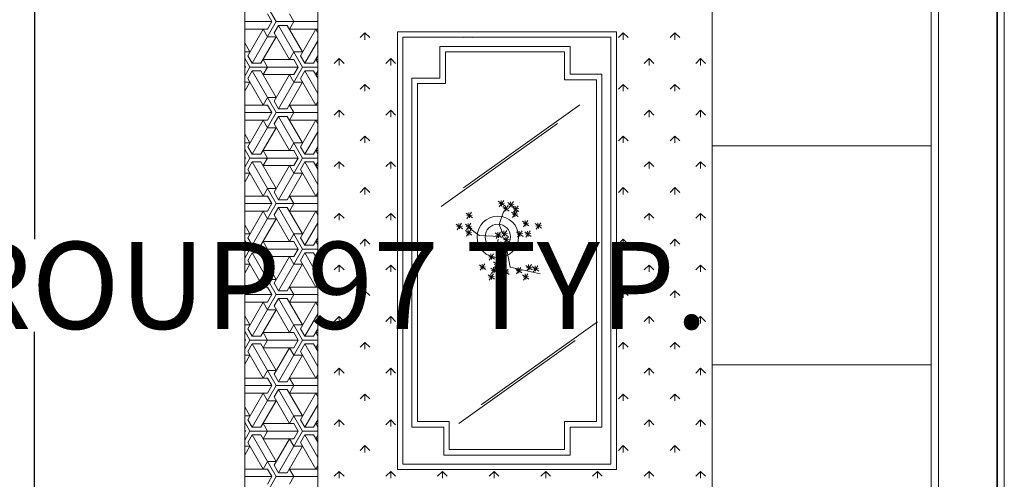
# Model space of a CAD drawing. Units: inches. Extents: x -1198 to -69, y -512 to 437.
# Tile 45 of 50: x -444 to -376, y 45 to 77. Entities that reach past the tile are written whole.
import ezdxf

# ---------------------------------------------------------------- set-up
doc = ezdxf.new("R2010")
doc.units = ezdxf.units.IN
doc.header["$MEASUREMENT"] = 0
for name, color, linetype, lineweight in [('A-ANNO-DIMS', 2, 'Continuous', 18), ('A-FURN', 60, 'Continuous', 18), ('A-WALL', 7, 'Continuous', 35)]:
    doc.layers.add(name, color=color, linetype=linetype, lineweight=lineweight)
doc.styles.get("Standard").update_dxf_attribs({"font": 'arial.ttf'})
doc.dimstyles.get("Standard").update_dxf_attribs({"dimtxt": 6, "dimasz": 6, "dimexe": 0.18, "dimexo": 0.0625, "dimgap": 0.09, "dimtad": 0, "dimtih": 1, "dimtoh": 1, "dimdec": 0, "dimzin": 0, "dimdsep": 46, "dimlunit": 4, "dimtxsty": 'Standard', "dimblk": 'OBLIQUE', "dimcen": 0.09, "dimadec": 0, "dimazin": 0, "dimtfac": 1, "dimtdec": 0, "dimtofl": 0, "dimtmove": 0, "dimatfit": 3, "dimfxl": 1, "dimtolj": 1, "dimtzin": 0, "dimarcsym": 0})

# ---------------------------------------------------------------- blocks, each defined once
blk = doc.blocks.new('A$C3B9F700E')
for p, q in [((736.9, 2080, -685.7), (2936.9, 2080, -685.7)), ((756.9, 2060, -685.7), (2916.9, 2060, -685.7)), ((2916.9, 1900, -685.7), (756.9, 1900, -685.7)), ((2936.9, 1880, -685.7), (736.9, 1880, -685.7)), ((2936.9, 1880, -685.7), (736.9, 1880, -685.7)), ((1536.9, 1880, -685.7), (1536.9, 1280, -685.7)), ((2136.9, 1880, -685.7), (2136.9, 1280, -685.7)), ((2736.9, 1280, -685.7), (936.9, 1280, -685.7)), ((1297.5, 1248.4, -685.7), (1310.8, 1261.7, -685.7)), ((1297.5, 1248.4, -685.7), (1310.8, 1235.2, -685.7)), ((1297.5, 1248.4, -685.7), (1316.3, 1248.4, -685.7)), ((1439, 1248.4, -685.7), (1452.2, 1261.7, -685.7)), ((1439, 1248.4, -685.7), (1452.2, 1235.2, -685.7)), ((1439, 1248.4, -685.7), (1457.7, 1248.4, -685.7)), ((1580.4, 1248.4, -685.7), (1593.6, 1261.7, -685.7)), ((1580.4, 1248.4, -685.7), (1593.6, 1235.2, -685.7)), ((1580.4, 1248.4, -685.7), (1599.1, 1248.4, -685.7)), ((1721.8, 1248.4, -685.7), (1735.1, 1261.7, -685.7)), ((1721.8, 1248.4, -685.7), (1735.1, 1235.2, -685.7)), ((1721.8, 1248.4, -685.7), (1740.6, 1248.4, -685.7)), ((1863.2, 1248.4, -685.7), (1876.5, 1261.7, -685.7)), ((1863.2, 1248.4, -685.7), (1876.5, 1235.2, -685.7)), ((1863.2, 1248.4, -685.7), (1882, 1248.4, -685.7)), ((2004.7, 1248.4, -685.7), (2017.9, 1261.7, -685.7)), ((2004.7, 1248.4, -685.7), (2017.9, 1235.2, -685.7)), ((2004.7, 1248.4, -685.7), (2023.4, 1248.4, -685.7)), ((2146.1, 1248.4, -685.7), (2159.3, 1261.7, -685.7)), ((2146.1, 1248.4, -685.7), (2159.3, 1235.2, -685.7)), ((2146.1, 1248.4, -685.7), (2164.8, 1248.4, -685.7)), ((2287.5, 1248.4, -685.7), (2300.8, 1261.7, -685.7)), ((2287.5, 1248.4, -685.7), (2300.8, 1235.2, -685.7)), ((2287.5, 1248.4, -685.7), (2306.2, 1248.4, -685.7)), ((2428.9, 1248.4, -685.7), (2442.2, 1261.7, -685.7)), ((2428.9, 1248.4, -685.7), (2442.2, 1235.2, -685.7)), ((2428.9, 1248.4, -685.7), (2447.7, 1248.4, -685.7)), ((1226.8, 1177.7, -685.7), (1240.1, 1191, -685.7)), ((1368.3, 1177.7, -685.7), (1381.5, 1191, -685.7)), ((1509.7, 1177.7, -685.7), (1522.9, 1191, -685.7)), ((1651.1, 1177.7, -685.7), (1664.4, 1191, -685.7)), ((1792.5, 1177.7, -685.7), (1805.8, 1191, -685.7)), ((1933.9, 1177.7, -685.7), (1947.2, 1191, -685.7)), ((2075.4, 1177.7, -685.7), (2088.6, 1191, -685.7)), ((2216.8, 1177.7, -685.7), (2230, 1191, -685.7)), ((2358.2, 1177.7, -685.7), (2371.5, 1191, -685.7)), ((1226.8, 1177.7, -685.7), (1240.1, 1164.5, -685.7)), ((1226.8, 1177.7, -685.7), (1245.6, 1177.7, -685.7)), ((1368.3, 1177.7, -685.7), (1381.5, 1164.5, -685.7)), ((1368.3, 1177.7, -685.7), (1387, 1177.7, -685.7)), ((1509.7, 1177.7, -685.7), (1522.9, 1164.5, -685.7)), ((1509.7, 1177.7, -685.7), (1528.4, 1177.7, -685.7)), ((1651.1, 1177.7, -685.7), (1664.4, 1164.5, -685.7)), ((1651.1, 1177.7, -685.7), (1669.9, 1177.7, -685.7)), ((1792.5, 1177.7, -685.7), (1805.8, 1164.5, -685.7)), ((1792.5, 1177.7, -685.7), (1811.3, 1177.7, -685.7)), ((1933.9, 1177.7, -685.7), (1947.2, 1164.5, -685.7)), ((1933.9, 1177.7, -685.7), (1952.7, 1177.7, -685.7)), ((2075.4, 1177.7, -685.7), (2088.6, 1164.5, -685.7)), ((2075.4, 1177.7, -685.7), (2094.1, 1177.7, -685.7)), ((2216.8, 1177.7, -685.7), (2230, 1164.5, -685.7)), ((2216.8, 1177.7, -685.7), (2235.5, 1177.7, -685.7)), ((2358.2, 1177.7, -685.7), (2371.5, 1164.5, -685.7)), ((2358.2, 1177.7, -685.7), (2377, 1177.7, -685.7)), ((1297.5, 1107, -685.7), (1310.8, 1120.3, -685.7)), ((1297.5, 1107, -685.7), (1310.8, 1093.8, -685.7)), ((1297.5, 1107, -685.7), (1316.3, 1107, -685.7)), ((1439, 1107, -685.7), (1452.2, 1120.3, -685.7)), ((1439, 1107, -685.7), (1452.2, 1093.8, -685.7)), ((1439, 1107, -685.7), (1457.7, 1107, -685.7)), ((1580.4, 1107, -685.7), (1593.6, 1120.3, -685.7)), ((1580.4, 1107, -685.7), (1593.6, 1093.8, -685.7)), ((1580.4, 1107, -685.7), (1599.1, 1107, -685.7)), ((1721.8, 1107, -685.7), (1735.1, 1120.3, -685.7)), ((1721.8, 1107, -685.7), (1735.1, 1093.8, -685.7)), ((1721.8, 1107, -685.7), (1740.6, 1107, -685.7)), ((1863.2, 1107, -685.7), (1876.5, 1120.3, -685.7)), ((1863.2, 1107, -685.7), (1876.5, 1093.8, -685.7)), ((1863.2, 1107, -685.7), (1882, 1107, -685.7)), ((2004.7, 1107, -685.7), (2017.9, 1120.3, -685.7)), ((2004.7, 1107, -685.7), (2017.9, 1093.8, -685.7)), ((2004.7, 1107, -685.7), (2023.4, 1107, -685.7)), ((2146.1, 1107, -685.7), (2159.3, 1120.3, -685.7)), ((2146.1, 1107, -685.7), (2159.3, 1093.8, -685.7)), ((2146.1, 1107, -685.7), (2164.8, 1107, -685.7)), ((2287.5, 1107, -685.7), (2300.8, 1120.3, -685.7)), ((2287.5, 1107, -685.7), (2300.8, 1093.8, -685.7)), ((2287.5, 1107, -685.7), (2306.2, 1107, -685.7)), ((2428.9, 1107, -685.7), (2442.2, 1120.3, -685.7)), ((2428.9, 1107, -685.7), (2442.2, 1093.8, -685.7)), ((2428.9, 1107, -685.7), (2447.7, 1107, -685.7)), ((1226.8, 1036.3, -685.7), (1240.1, 1049.6, -685.7)), ((1226.8, 1036.3, -685.7), (1240.1, 1023.1, -685.7)), ((1226.8, 1036.3, -685.7), (1245.6, 1036.3, -685.7)), ((1368.3, 1036.3, -685.7), (1381.5, 1049.6, -685.7)), ((1368.3, 1036.3, -685.7), (1381.5, 1023.1, -685.7)), ((1368.3, 1036.3, -685.7), (1387, 1036.3, -685.7)), ((1509.7, 1036.3, -685.7), (1522.9, 1049.6, -685.7)), ((1509.7, 1036.3, -685.7), (1522.9, 1023.1, -685.7)), ((1509.7, 1036.3, -685.7), (1528.4, 1036.3, -685.7)), ((1651.1, 1036.3, -685.7), (1664.4, 1049.6, -685.7)), ((1651.1, 1036.3, -685.7), (1664.4, 1023.1, -685.7)), ((1651.1, 1036.3, -685.7), (1669.9, 1036.3, -685.7)), ((1792.5, 1036.3, -685.7), (1805.8, 1049.6, -685.7)), ((1792.5, 1036.3, -685.7), (1805.8, 1023.1, -685.7)), ((1792.5, 1036.3, -685.7), (1811.3, 1036.3, -685.7)), ((1933.9, 1036.3, -685.7), (1947.2, 1049.6, -685.7)), ((1933.9, 1036.3, -685.7), (1947.2, 1023.1, -685.7)), ((1933.9, 1036.3, -685.7), (1952.7, 1036.3, -685.7)), ((2075.4, 1036.3, -685.7), (2088.6, 1049.6, -685.7)), ((2075.4, 1036.3, -685.7), (2088.6, 1023.1, -685.7)), ((2075.4, 1036.3, -685.7), (2094.1, 1036.3, -685.7)), ((2216.8, 1036.3, -685.7), (2230, 1049.6, -685.7)), ((2216.8, 1036.3, -685.7), (2230, 1023.1, -685.7)), ((2216.8, 1036.3, -685.7), (2235.5, 1036.3, -685.7)), ((2358.2, 1036.3, -685.7), (2371.5, 1049.6, -685.7)), ((2358.2, 1036.3, -685.7), (2371.5, 1023.1, -685.7)), ((2358.2, 1036.3, -685.7), (2377, 1036.3, -685.7)), ((1224, 417.9, -685.7), (1224, 1017.9, -685.7)), ((1224, 1017.9, -685.7), (2424, 1017.9, -685.7)), ((1239, 432.9, -685.7), (1239, 1002.9, -685.7)), ((1239, 1002.9, -685.7), (2409, 1002.9, -685.7)), ((2409, 1002.9, -685.7), (2409, 432.9, -685.7)), ((2424, 1017.9, -685.7), (2424, 417.9, -685.7)), ((1340.5, 977.9, -685.7), (2307.5, 977.9, -685.7)), ((1340.5, 890.9, -685.7), (1340.5, 977.9, -685.7)), ((2307.5, 977.9, -685.7), (2307.5, 890.9, -685.7)), ((2428.9, 965.6, -685.7), (2442.2, 978.9, -685.7)), ((1355.5, 962.9, -685.7), (2292.5, 962.9, -685.7)), ((1355.5, 875.9, -685.7), (1355.5, 962.9, -685.7)), ((2246, 647.2, -685.7), (2018.6, 965.9, -685.7)), ((2292.5, 962.9, -685.7), (2292.5, 875.9, -685.7)), ((2428.9, 965.6, -685.7), (2442.2, 952.3, -685.7)), ((2428.9, 965.6, -685.7), (2447.7, 965.6, -685.7)), ((1651.7, 598.7, -685.7), (1424.3, 917.3, -685.7)), ((1264, 534.4, -685.7), (1264, 890.9, -685.7)), ((1264, 890.9, -685.7), (1340.5, 890.9, -685.7)), ((2297.5, 586.5, -685.7), (2070.1, 905.2, -685.7)), ((2307.5, 890.9, -685.7), (2384, 890.9, -685.7)), ((2384, 890.9, -685.7), (2384, 544.9, -685.7)), ((1279, 549.4, -685.7), (1279, 875.9, -685.7)), ((1279, 875.9, -685.7), (1355.5, 875.9, -685.7)), ((2292.5, 875.9, -685.7), (2369, 875.9, -685.7)), ((2369, 875.9, -685.7), (2369, 559.9, -685.7)), ((1703.2, 538, -685.7), (1475.8, 856.6, -685.7)), ((2428.9, 824.2, -685.7), (2442.2, 837.4, -685.7)), ((1764.8, 797.9, -685.7), (1747.3, 810.4, -685.7)), ((1762.3, 812.9, -685.7), (1749.8, 795.4, -685.7)), ((1756.5, 797.3, -685.7), (1754.9, 812.4, -685.7)), ((1869.5, 726.5, -685.7), (1887, 808.9, -685.7)), ((2428.9, 824.2, -685.7), (2442.2, 810.9, -685.7)), ((2428.9, 824.2, -685.7), (2447.7, 824.2, -685.7)), ((1762.8, 804.4, -685.7), (1747.7, 802.8, -685.7)), ((1784.6, 784.3, -685.7), (1772.1, 766.8, -685.7)), ((1778.7, 768.6, -685.7), (1777.1, 783.7, -685.7)), ((1879.3, 772.4, -685.7), (1861.8, 784.9, -685.7)), ((1876.8, 787.4, -685.7), (1864.3, 769.9, -685.7)), ((1882.5, 790, -685.7), (1865, 802.5, -685.7)), ((1880.5, 796.5, -685.7), (1865.4, 794.9, -685.7)), ((1880, 805, -685.7), (1867.5, 787.5, -685.7)), ((1871, 771.8, -685.7), (1869.4, 786.9, -685.7)), ((1874.2, 789.3, -685.7), (1872.6, 804.4, -685.7)), ((1758.4, 762.9, -685.7), (1741, 775.4, -685.7)), ((1756.5, 769.4, -685.7), (1741.3, 767.8, -685.7)), ((1755.9, 777.9, -685.7), (1743.4, 760.4, -685.7)), ((1750.1, 762.2, -685.7), (1748.5, 777.4, -685.7)), ((1787.1, 769.3, -685.7), (1769.6, 781.8, -685.7)), ((1787.1, 747, -685.7), (1769.6, 759.5, -685.7)), ((1785.1, 775.8, -685.7), (1770, 774.2, -685.7)), ((1784.6, 762, -685.7), (1772.1, 744.5, -685.7)), ((1778.7, 746.3, -685.7), (1777.1, 761.4, -685.7)), ((1877.4, 779, -685.7), (1862.2, 777.4, -685.7)), ((1887.3, 743.8, -685.7), (1869.8, 756.3, -685.7)), ((1884.8, 758.8, -685.7), (1872.3, 741.3, -685.7)), ((1878.9, 743.1, -685.7), (1877.4, 758.3, -685.7)), ((1904.8, 762.9, -685.7), (1887.3, 775.4, -685.7)), ((1902.8, 769.4, -685.7), (1887.7, 767.8, -685.7)), ((1902.3, 777.9, -685.7), (1889.8, 760.4, -685.7)), ((1896.4, 762.2, -685.7), (1894.9, 777.4, -685.7)), ((1706.7, 723.1, -685.7), (1689.3, 735.6, -685.7)), ((1704.8, 729.6, -685.7), (1689.6, 728, -685.7)), ((1704.2, 738.1, -685.7), (1691.7, 720.6, -685.7)), ((1698.4, 722.4, -685.7), (1696.8, 737.6, -685.7)), ((1718.7, 735.8, -685.7), (1701.2, 748.3, -685.7)), ((1716.7, 742.3, -685.7), (1701.6, 740.7, -685.7)), ((1716.2, 750.8, -685.7), (1703.7, 733.3, -685.7)), ((1710.3, 735.2, -685.7), (1708.7, 750.3, -685.7)), ((1733, 733.4, -685.7), (1715.5, 745.9, -685.7)), ((1731, 740, -685.7), (1715.9, 738.4, -685.7)), ((1730.5, 748.4, -685.7), (1718, 730.9, -685.7)), ((1724.6, 732.8, -685.7), (1723.1, 747.9, -685.7)), ((1785.1, 753.5, -685.7), (1770, 751.9, -685.7)), ((1885.3, 750.3, -685.7), (1870.2, 748.7, -685.7)), ((1703.5, 696.8, -685.7), (1686.1, 709.3, -685.7)), ((1701.6, 703.3, -685.7), (1686.5, 701.7, -685.7)), ((1701, 711.8, -685.7), (1688.6, 694.3, -685.7)), ((1695.2, 696.2, -685.7), (1693.6, 711.3, -685.7)), ((1717.9, 708.8, -685.7), (1700.4, 721.3, -685.7)), ((1715.9, 715.3, -685.7), (1700.8, 713.7, -685.7)), ((1715.4, 723.8, -685.7), (1702.9, 706.3, -685.7)), ((1709.5, 708.1, -685.7), (1707.9, 723.2, -685.7)), ((1752.2, 696.5, -685.7), (1717.2, 709, -685.7)), ((1777.1, 706.5, -685.7), (1752.2, 696.5, -685.7)), ((1786.3, 704.8, -685.7), (1768.8, 717.3, -685.7)), ((1784.3, 711.3, -685.7), (1769.2, 709.7, -685.7)), ((1783.8, 719.8, -685.7), (1771.3, 702.3, -685.7)), ((1787.7, 703.1, -685.7), (1775.3, 685.6, -685.7)), ((1777.9, 704.1, -685.7), (1776.3, 719.3, -685.7)), ((1781.9, 687.4, -685.7), (1780.3, 702.5, -685.7)), ((1803, 709.6, -685.7), (1785.5, 722, -685.7)), ((1801, 716.1, -685.7), (1785.9, 714.5, -685.7)), ((1800.5, 724.5, -685.7), (1788, 707.1, -685.7)), ((1794.6, 708.9, -685.7), (1793, 724, -685.7)), ((1817.3, 689.7, -685.7), (1799.8, 702.1, -685.7)), ((1802.1, 714, -685.7), (1869.5, 726.5, -685.7)), ((1814.8, 704.6, -685.7), (1802.3, 687.2, -685.7)), ((1809, 689, -685.7), (1807.4, 704.1, -685.7)), ((1824.6, 689, -685.7), (1872, 714, -685.7)), ((1892, 708.8, -685.7), (1874.6, 721.3, -685.7)), ((1890.1, 715.3, -685.7), (1875, 713.7, -685.7)), ((1889.6, 723.8, -685.7), (1877.1, 706.3, -685.7)), ((1883.7, 708.1, -685.7), (1882.1, 723.2, -685.7)), ((1790.2, 688.1, -685.7), (1772.8, 700.6, -685.7)), ((1788.3, 694.6, -685.7), (1773.2, 693, -685.7)), ((1784.6, 699, -685.7), (1782.1, 641.6, -685.7)), ((1792.1, 694, -685.7), (1824.6, 689, -685.7)), ((1815.3, 696.2, -685.7), (1800.2, 694.6, -685.7)), ((1849.9, 669, -685.7), (1832.4, 681.5, -685.7)), ((1847.9, 675.5, -685.7), (1832.8, 673.9, -685.7)), ((1847.4, 683.9, -685.7), (1834.9, 666.5, -685.7)), ((1841.6, 668.3, -685.7), (1840, 683.4, -685.7)), ((1869.8, 684.1, -685.7), (1852.3, 696.6, -685.7)), ((1867.8, 690.6, -685.7), (1852.7, 689, -685.7)), ((1867.3, 699.1, -685.7), (1854.8, 681.6, -685.7)), ((1861.4, 683.4, -685.7), (1859.9, 698.6, -685.7)), ((1886.5, 676.1, -685.7), (1869, 688.6, -685.7)), ((1884.5, 682.6, -685.7), (1869.4, 681, -685.7)), ((1884, 691.1, -685.7), (1871.5, 673.6, -685.7)), ((1878.1, 675.5, -685.7), (1876.6, 690.6, -685.7)), ((1904.8, 669, -685.7), (1887.3, 681.5, -685.7)), ((1902.8, 675.5, -685.7), (1887.7, 673.9, -685.7)), ((1902.3, 683.9, -685.7), (1889.8, 666.5, -685.7)), ((1896.4, 668.3, -685.7), (1894.9, 683.4, -685.7)), ((2428.9, 682.8, -685.7), (2442.2, 696, -685.7)), ((2428.9, 682.8, -685.7), (2442.2, 669.5, -685.7)), ((2428.9, 682.8, -685.7), (2447.7, 682.8, -685.7)), ((1877.7, 645.1, -685.7), (1860.3, 657.6, -685.7)), ((1875.8, 651.6, -685.7), (1860.7, 650, -685.7)), ((1875.2, 660.1, -685.7), (1862.8, 642.6, -685.7)), ((1869.4, 644.4, -685.7), (1867.8, 659.5, -685.7)), ((1239, 624.2, -685.7), (1240.1, 625.3, -685.7)), ((1736.2, 608.5, -685.7), (1718.7, 621, -685.7)), ((1733.7, 623.4, -685.7), (1721.2, 606, -685.7)), ((1727.8, 607.8, -685.7), (1726.2, 622.9, -685.7)), ((1763.9, 621.9, -685.7), (1751.4, 604.4, -685.7)), ((1758, 606.2, -685.7), (1756.5, 621.3, -685.7)), ((1782.1, 641.6, -685.7), (1759.7, 611.6, -685.7)), ((1781.4, 621.9, -685.7), (1768.9, 604.4, -685.7)), ((1775.5, 606.2, -685.7), (1774, 621.3, -685.7)), ((1239, 599.9, -685.7), (1240.1, 598.8, -685.7)), ((1734.2, 615, -685.7), (1719.1, 613.4, -685.7)), ((1766.4, 606.9, -685.7), (1748.9, 619.4, -685.7)), ((1766.4, 581.4, -685.7), (1748.9, 593.9, -685.7)), ((1764.4, 613.4, -685.7), (1749.3, 611.8, -685.7)), ((1763.9, 596.4, -685.7), (1751.4, 578.9, -685.7)), ((1758, 580.7, -685.7), (1756.5, 595.9, -685.7)), ((1783.9, 606.9, -685.7), (1766.4, 619.4, -685.7)), ((1781.9, 613.4, -685.7), (1766.8, 611.8, -685.7)), ((1764.4, 587.9, -685.7), (1749.3, 586.3, -685.7)), ((1366, 549.4, -685.7), (1279, 549.4, -685.7)), ((1366, 472.9, -685.7), (1366, 549.4, -685.7)), ((2292.5, 559.9, -685.7), (2292.5, 472.9, -685.7)), ((2369, 559.9, -685.7), (2292.5, 559.9, -685.7)), ((2307.5, 544.9, -685.7), (2307.5, 457.9, -685.7)), ((2384, 544.9, -685.7), (2307.5, 544.9, -685.7)), ((2428.9, 541.3, -685.7), (2442.2, 554.6, -685.7)), ((2428.9, 541.3, -685.7), (2442.2, 528.1, -685.7)), ((2428.9, 541.3, -685.7), (2447.7, 541.3, -685.7)), ((1351, 534.4, -685.7), (1264, 534.4, -685.7)), ((1351, 457.9, -685.7), (1351, 534.4, -685.7)), ((2292.5, 472.9, -685.7), (1366, 472.9, -685.7)), ((2409, 432.9, -685.7), (1239, 432.9, -685.7)), ((2307.5, 457.9, -685.7), (1351, 457.9, -685.7)), ((2424, 417.9, -685.7), (1224, 417.9, -685.7)), ((1297.5, 399.9, -685.7), (1310.8, 413.2, -685.7)), ((1439, 399.9, -685.7), (1452.2, 413.2, -685.7)), ((1580.4, 399.9, -685.7), (1593.6, 413.2, -685.7)), ((1721.8, 399.9, -685.7), (1735.1, 413.2, -685.7)), ((1863.2, 399.9, -685.7), (1876.5, 413.2, -685.7)), ((2004.7, 399.9, -685.7), (2017.9, 413.2, -685.7)), ((2146.1, 399.9, -685.7), (2159.3, 413.2, -685.7)), ((2287.5, 399.9, -685.7), (2300.8, 413.2, -685.7)), ((2428.9, 399.9, -685.7), (2442.2, 413.2, -685.7)), ((1297.5, 399.9, -685.7), (1316.3, 399.9, -685.7)), ((1297.5, 399.9, -685.7), (1310.8, 386.7, -685.7)), ((1439, 399.9, -685.7), (1457.7, 399.9, -685.7)), ((1439, 399.9, -685.7), (1452.2, 386.7, -685.7)), ((1580.4, 399.9, -685.7), (1599.1, 399.9, -685.7)), ((1580.4, 399.9, -685.7), (1593.6, 386.7, -685.7)), ((1721.8, 399.9, -685.7), (1740.6, 399.9, -685.7)), ((1721.8, 399.9, -685.7), (1735.1, 386.7, -685.7)), ((1863.2, 399.9, -685.7), (1882, 399.9, -685.7)), ((1863.2, 399.9, -685.7), (1876.5, 386.7, -685.7)), ((2004.7, 399.9, -685.7), (2023.4, 399.9, -685.7)), ((2004.7, 399.9, -685.7), (2017.9, 386.7, -685.7)), ((2146.1, 399.9, -685.7), (2164.8, 399.9, -685.7)), ((2146.1, 399.9, -685.7), (2159.3, 386.7, -685.7)), ((2287.5, 399.9, -685.7), (2306.2, 399.9, -685.7)), ((2287.5, 399.9, -685.7), (2300.8, 386.7, -685.7)), ((2428.9, 399.9, -685.7), (2447.7, 399.9, -685.7)), ((2428.9, 399.9, -685.7), (2442.2, 386.7, -685.7)), ((1226.8, 329.2, -685.7), (1240.1, 342.5, -685.7)), ((1226.8, 329.2, -685.7), (1240.1, 315.9, -685.7)), ((1226.8, 329.2, -685.7), (1245.6, 329.2, -685.7)), ((1368.3, 329.2, -685.7), (1381.5, 342.5, -685.7)), ((1368.3, 329.2, -685.7), (1381.5, 315.9, -685.7)), ((1368.3, 329.2, -685.7), (1387, 329.2, -685.7)), ((1509.7, 329.2, -685.7), (1522.9, 342.5, -685.7)), ((1509.7, 329.2, -685.7), (1522.9, 315.9, -685.7)), ((1509.7, 329.2, -685.7), (1528.4, 329.2, -685.7)), ((1651.1, 329.2, -685.7), (1664.4, 342.5, -685.7)), ((1651.1, 329.2, -685.7), (1664.4, 315.9, -685.7)), ((1651.1, 329.2, -685.7), (1669.9, 329.2, -685.7)), ((1792.5, 329.2, -685.7), (1805.8, 342.5, -685.7)), ((1792.5, 329.2, -685.7), (1805.8, 315.9, -685.7)), ((1792.5, 329.2, -685.7), (1811.3, 329.2, -685.7)), ((1933.9, 329.2, -685.7), (1947.2, 342.5, -685.7)), ((1933.9, 329.2, -685.7), (1947.2, 315.9, -685.7)), ((1933.9, 329.2, -685.7), (1952.7, 329.2, -685.7)), ((2075.4, 329.2, -685.7), (2088.6, 342.5, -685.7)), ((2075.4, 329.2, -685.7), (2088.6, 315.9, -685.7)), ((2075.4, 329.2, -685.7), (2094.1, 329.2, -685.7)), ((2216.8, 329.2, -685.7), (2230, 342.5, -685.7)), ((2216.8, 329.2, -685.7), (2230, 315.9, -685.7)), ((2216.8, 329.2, -685.7), (2235.5, 329.2, -685.7)), ((2358.2, 329.2, -685.7), (2371.5, 342.5, -685.7)), ((2358.2, 329.2, -685.7), (2371.5, 315.9, -685.7)), ((2358.2, 329.2, -685.7), (2377, 329.2, -685.7)), ((1297.5, 258.5, -685.7), (1310.8, 271.8, -685.7)), ((1439, 258.5, -685.7), (1452.2, 271.8, -685.7)), ((1580.4, 258.5, -685.7), (1593.6, 271.8, -685.7)), ((1721.8, 258.5, -685.7), (1735.1, 271.8, -685.7)), ((1863.2, 258.5, -685.7), (1876.5, 271.8, -685.7)), ((2004.7, 258.5, -685.7), (2017.9, 271.8, -685.7)), ((2146.1, 258.5, -685.7), (2159.3, 271.8, -685.7)), ((2287.5, 258.5, -685.7), (2300.8, 271.8, -685.7)), ((2428.9, 258.5, -685.7), (2442.2, 271.8, -685.7)), ((1297.5, 258.5, -685.7), (1310.8, 245.2, -685.7)), ((1297.5, 258.5, -685.7), (1316.3, 258.5, -685.7)), ((1439, 258.5, -685.7), (1452.2, 245.2, -685.7)), ((1439, 258.5, -685.7), (1457.7, 258.5, -685.7)), ((1580.4, 258.5, -685.7), (1593.6, 245.2, -685.7)), ((1580.4, 258.5, -685.7), (1599.1, 258.5, -685.7)), ((1721.8, 258.5, -685.7), (1735.1, 245.2, -685.7)), ((1721.8, 258.5, -685.7), (1740.6, 258.5, -685.7)), ((1863.2, 258.5, -685.7), (1876.5, 245.2, -685.7)), ((1863.2, 258.5, -685.7), (1882, 258.5, -685.7)), ((2004.7, 258.5, -685.7), (2017.9, 245.2, -685.7)), ((2004.7, 258.5, -685.7), (2023.4, 258.5, -685.7)), ((2146.1, 258.5, -685.7), (2159.3, 245.2, -685.7)), ((2146.1, 258.5, -685.7), (2164.8, 258.5, -685.7)), ((2287.5, 258.5, -685.7), (2300.8, 245.2, -685.7)), ((2287.5, 258.5, -685.7), (2306.2, 258.5, -685.7)), ((2428.9, 258.5, -685.7), (2442.2, 245.2, -685.7)), ((2428.9, 258.5, -685.7), (2447.7, 258.5, -685.7)), ((3062.1, 200, -685.7), (601.4, 200, -685.7)), ((3062.1, 200, -685.7), (601.4, 200, -685.7)), ((1196, 86.3, -685.7), (1196, 200, -685.7)), ((1216.8, 200, -685.7), (1216.8, 122.3, -685.7)), ((1226.6, 200, -685.7), (1216.8, 194.3, -685.7)), ((1289.6, 152.3, -685.7), (1216.8, 194.3, -685.7)), ((1239.1, 200, -685.7), (1240.1, 201, -685.7)), ((1248.5, 200, -685.7), (1310.3, 164.3, -685.7)), ((1310.3, 188.3, -685.7), (1290.1, 200, -685.7)), ((1299.9, 200, -685.7), (1299.9, 194.3, -685.7)), ((1309.8, 200, -685.7), (1299.9, 194.3, -685.7)), ((1320.7, 158.3, -685.7), (1320.7, 200, -685.7)), ((1331.1, 188.3, -685.7), (1351.3, 200, -685.7)), ((1392.9, 200, -685.7), (1331.1, 164.3, -685.7)), ((1331.7, 200, -685.7), (1341.5, 194.3, -685.7)), ((1341.5, 200, -685.7), (1341.5, 194.3, -685.7)), ((1351.9, 152.3, -685.7), (1424.7, 194.3, -685.7)), ((1380.5, 200, -685.7), (1381.5, 201, -685.7)), ((1414.8, 200, -685.7), (1424.7, 194.3, -685.7)), ((1424.7, 200, -685.7), (1424.7, 122.3, -685.7)), ((1445.4, 86.3, -685.7), (1445.4, 200, -685.7)), ((1466.2, 200, -685.7), (1466.2, 122.3, -685.7)), ((1476.1, 200, -685.7), (1466.2, 194.3, -685.7)), ((1539, 152.3, -685.7), (1466.2, 194.3, -685.7)), ((1498, 200, -685.7), (1559.8, 164.3, -685.7)), ((1521.9, 200, -685.7), (1522.9, 201, -685.7)), ((1559.8, 188.3, -685.7), (1539.5, 200, -685.7)), ((1549.4, 200, -685.7), (1549.4, 194.3, -685.7)), ((1559.2, 200, -685.7), (1549.4, 194.3, -685.7)), ((1570.1, 158.3, -685.7), (1570.1, 200, -685.7)), ((1580.5, 188.3, -685.7), (1600.8, 200, -685.7)), ((1642.3, 200, -685.7), (1580.5, 164.3, -685.7)), ((1581.1, 200, -685.7), (1590.9, 194.3, -685.7)), ((1590.9, 200, -685.7), (1590.9, 194.3, -685.7)), ((1601.3, 152.3, -685.7), (1674.1, 194.3, -685.7)), ((1663.3, 200, -685.7), (1664.4, 201, -685.7)), ((1664.2, 200, -685.7), (1674.1, 194.3, -685.7)), ((1674.1, 200, -685.7), (1674.1, 122.3, -685.7)), ((1694.9, 86.3, -685.7), (1694.9, 200, -685.7)), ((1715.6, 200, -685.7), (1715.6, 122.3, -685.7)), ((1725.5, 200, -685.7), (1715.6, 194.3, -685.7)), ((1788.4, 152.3, -685.7), (1715.6, 194.3, -685.7)), ((1747.4, 200, -685.7), (1809.2, 164.3, -685.7)), ((1809.2, 188.3, -685.7), (1788.9, 200, -685.7)), ((1798.8, 200, -685.7), (1798.8, 194.3, -685.7)), ((1808.6, 200, -685.7), (1798.8, 194.3, -685.7)), ((1804.7, 200, -685.7), (1805.8, 201, -685.7)), ((1819.6, 158.3, -685.7), (1819.6, 200, -685.7)), ((1830, 188.3, -685.7), (1850.2, 200, -685.7)), ((1891.7, 200, -685.7), (1830, 164.3, -685.7)), ((1830.5, 200, -685.7), (1840.3, 194.3, -685.7)), ((1840.3, 200, -685.7), (1840.3, 194.3, -685.7)), ((1850.7, 152.3, -685.7), (1923.5, 194.3, -685.7)), ((1913.6, 200, -685.7), (1923.5, 194.3, -685.7)), ((1923.5, 200, -685.7), (1923.5, 122.3, -685.7)), ((1944.3, 86.3, -685.7), (1944.3, 200, -685.7)), ((1946.2, 200, -685.7), (1947.2, 201, -685.7)), ((1965.1, 200, -685.7), (1965.1, 122.3, -685.7)), ((1974.9, 200, -685.7), (1965.1, 194.3, -685.7)), ((2037.8, 152.3, -685.7), (1965.1, 194.3, -685.7)), ((1996.8, 200, -685.7), (2058.6, 164.3, -685.7)), ((2058.6, 188.3, -685.7), (2038.4, 200, -685.7)), ((2048.2, 200, -685.7), (2048.2, 194.3, -685.7)), ((2058, 200, -685.7), (2048.2, 194.3, -685.7)), ((2069, 158.3, -685.7), (2069, 200, -685.7)), ((2079.4, 188.3, -685.7), (2099.6, 200, -685.7)), ((2141.2, 200, -685.7), (2079.4, 164.3, -685.7)), ((2079.9, 200, -685.7), (2089.8, 194.3, -685.7)), ((2087.6, 200, -685.7), (2088.6, 201, -685.7)), ((2089.8, 200, -685.7), (2089.8, 194.3, -685.7)), ((2100.2, 152.3, -685.7), (2172.9, 194.3, -685.7)), ((2163.1, 200, -685.7), (2172.9, 194.3, -685.7)), ((2172.9, 200, -685.7), (2172.9, 122.3, -685.7)), ((2193.7, 86.3, -685.7), (2193.7, 200, -685.7)), ((2214.5, 200, -685.7), (2214.5, 122.3, -685.7)), ((2224.3, 200, -685.7), (2214.5, 194.3, -685.7)), ((2287.2, 152.3, -685.7), (2214.5, 194.3, -685.7)), ((2229, 200, -685.7), (2230, 201, -685.7)), ((2246.2, 200, -685.7), (2308, 164.3, -685.7)), ((2308, 188.3, -685.7), (2287.8, 200, -685.7)), ((2297.6, 200, -685.7), (2297.6, 194.3, -685.7)), ((2307.4, 200, -685.7), (2297.6, 194.3, -685.7)), ((2318.4, 158.3, -685.7), (2318.4, 200, -685.7)), ((2328.8, 188.3, -685.7), (2349, 200, -685.7)), ((2390.6, 200, -685.7), (2328.8, 164.3, -685.7)), ((2329.3, 200, -685.7), (2339.2, 194.3, -685.7)), ((2339.2, 200, -685.7), (2339.2, 194.3, -685.7)), ((2349.6, 152.3, -685.7), (2422.3, 194.3, -685.7)), ((2370.4, 200, -685.7), (2371.5, 201, -685.7)), ((2412.5, 200, -685.7), (2422.3, 194.3, -685.7)), ((2422.3, 200, -685.7), (2422.3, 122.3, -685.7)), ((2443.1, 86.3, -685.7), (2443.1, 200, -685.7)), ((1310.3, 164.3, -685.7), (1289.6, 152.3, -685.7)), ((1310.3, 164.3, -685.7), (1310.3, 188.3, -685.7)), ((1331.1, 164.3, -685.7), (1331.1, 188.3, -685.7)), ((1331.1, 164.3, -685.7), (1351.9, 152.3, -685.7)), ((1559.8, 164.3, -685.7), (1539, 152.3, -685.7)), ((1559.8, 164.3, -685.7), (1559.8, 188.3, -685.7)), ((1580.5, 164.3, -685.7), (1580.5, 188.3, -685.7)), ((1580.5, 164.3, -685.7), (1601.3, 152.3, -685.7)), ((1809.2, 164.3, -685.7), (1788.4, 152.3, -685.7)), ((1809.2, 164.3, -685.7), (1809.2, 188.3, -685.7)), ((1830, 164.3, -685.7), (1830, 188.3, -685.7)), ((1830, 164.3, -685.7), (1850.7, 152.3, -685.7)), ((2058.6, 164.3, -685.7), (2037.8, 152.3, -685.7)), ((2058.6, 164.3, -685.7), (2058.6, 188.3, -685.7)), ((2079.4, 164.3, -685.7), (2079.4, 188.3, -685.7)), ((2079.4, 164.3, -685.7), (2100.2, 152.3, -685.7)), ((2308, 164.3, -685.7), (2287.2, 152.3, -685.7)), ((2308, 164.3, -685.7), (2308, 188.3, -685.7)), ((2328.8, 164.3, -685.7), (2328.8, 188.3, -685.7)), ((2328.8, 164.3, -685.7), (2349.6, 152.3, -685.7)), ((1206.4, 116.3, -685.7), (1279.2, 158.3, -685.7)), ((1320.7, 158.3, -685.7), (1206.4, 92.3, -685.7)), ((1279.2, 134.3, -685.7), (1279.2, 158.3, -685.7)), ((1320.7, 146.3, -685.7), (1299.9, 134.3, -685.7)), ((1320.7, 158.3, -685.7), (1435, 92.3, -685.7)), ((1320.7, 146.3, -685.7), (1341.5, 134.3, -685.7)), ((1320.7, 14.3, -685.7), (1320.7, 146.3, -685.7)), ((1435, 116.3, -685.7), (1362.3, 158.3, -685.7)), ((1362.3, 134.3, -685.7), (1362.3, 158.3, -685.7)), ((1455.8, 116.3, -685.7), (1528.6, 158.3, -685.7)), ((1570.1, 158.3, -685.7), (1455.8, 92.3, -685.7)), ((1528.6, 134.3, -685.7), (1528.6, 158.3, -685.7)), ((1570.1, 146.3, -685.7), (1549.4, 134.3, -685.7)), ((1570.1, 158.3, -685.7), (1684.5, 92.3, -685.7)), ((1570.1, 146.3, -685.7), (1590.9, 134.3, -685.7)), ((1570.1, 14.3, -685.7), (1570.1, 146.3, -685.7)), ((1684.5, 116.3, -685.7), (1611.7, 158.3, -685.7)), ((1611.7, 134.3, -685.7), (1611.7, 158.3, -685.7)), ((1705.2, 116.3, -685.7), (1778, 158.3, -685.7)), ((1819.6, 158.3, -685.7), (1705.2, 92.3, -685.7)), ((1778, 134.3, -685.7), (1778, 158.3, -685.7)), ((1819.6, 146.3, -685.7), (1798.8, 134.3, -685.7)), ((1819.6, 158.3, -685.7), (1933.9, 92.3, -685.7)), ((1819.6, 146.3, -685.7), (1840.3, 134.3, -685.7)), ((1819.6, 14.3, -685.7), (1819.6, 146.3, -685.7)), ((1933.9, 116.3, -685.7), (1861.1, 158.3, -685.7)), ((1861.1, 134.3, -685.7), (1861.1, 158.3, -685.7)), ((1954.7, 116.3, -685.7), (2027.4, 158.3, -685.7)), ((2069, 158.3, -685.7), (1954.7, 92.3, -685.7)), ((2027.4, 134.3, -685.7), (2027.4, 158.3, -685.7)), ((2069, 146.3, -685.7), (2048.2, 134.3, -685.7)), ((2069, 158.3, -685.7), (2183.3, 92.3, -685.7)), ((2069, 146.3, -685.7), (2089.8, 134.3, -685.7)), ((2069, 14.3, -685.7), (2069, 146.3, -685.7)), ((2183.3, 116.3, -685.7), (2110.5, 158.3, -685.7)), ((2110.5, 134.3, -685.7), (2110.5, 158.3, -685.7)), ((2204.1, 116.3, -685.7), (2276.8, 158.3, -685.7)), ((2318.4, 158.3, -685.7), (2204.1, 92.3, -685.7)), ((2276.8, 134.3, -685.7), (2276.8, 158.3, -685.7)), ((2318.4, 146.3, -685.7), (2297.6, 134.3, -685.7)), ((2318.4, 158.3, -685.7), (2432.7, 92.3, -685.7)), ((2318.4, 146.3, -685.7), (2339.2, 134.3, -685.7)), ((2318.4, 14.3, -685.7), (2318.4, 146.3, -685.7)), ((2432.7, 116.3, -685.7), (2360, 158.3, -685.7)), ((2360, 134.3, -685.7), (2360, 158.3, -685.7)), ((1196, 134.3, -685.7), (1175.2, 122.3, -685.7)), ((1196, 134.3, -685.7), (1216.8, 122.3, -685.7)), ((1206.4, 92.3, -685.7), (1206.4, 116.3, -685.7)), ((1227.2, 80.3, -685.7), (1299.9, 122.3, -685.7)), ((1279.2, 134.3, -685.7), (1299.9, 122.3, -685.7)), ((1299.9, 134.3, -685.7), (1299.9, 50.3, -685.7)), ((1341.5, 134.3, -685.7), (1341.5, 50.3, -685.7)), ((1362.3, 134.3, -685.7), (1341.5, 122.3, -685.7)), ((1414.3, 80.3, -685.7), (1341.5, 122.3, -685.7)), ((1445.4, 134.3, -685.7), (1424.7, 122.3, -685.7)), ((1435, 92.3, -685.7), (1435, 116.3, -685.7)), ((1445.4, 134.3, -685.7), (1466.2, 122.3, -685.7)), ((1455.8, 92.3, -685.7), (1455.8, 116.3, -685.7)), ((1476.6, 80.3, -685.7), (1549.4, 122.3, -685.7)), ((1528.6, 134.3, -685.7), (1549.4, 122.3, -685.7)), ((1549.4, 134.3, -685.7), (1549.4, 50.3, -685.7)), ((1590.9, 134.3, -685.7), (1590.9, 50.3, -685.7)), ((1611.7, 134.3, -685.7), (1590.9, 122.3, -685.7)), ((1663.7, 80.3, -685.7), (1590.9, 122.3, -685.7)), ((1694.9, 134.3, -685.7), (1674.1, 122.3, -685.7)), ((1684.5, 92.3, -685.7), (1684.5, 116.3, -685.7)), ((1694.9, 134.3, -685.7), (1715.6, 122.3, -685.7)), ((1705.2, 92.3, -685.7), (1705.2, 116.3, -685.7)), ((1726, 80.3, -685.7), (1798.8, 122.3, -685.7)), ((1778, 134.3, -685.7), (1798.8, 122.3, -685.7)), ((1798.8, 134.3, -685.7), (1798.8, 50.3, -685.7)), ((1840.3, 134.3, -685.7), (1840.3, 50.3, -685.7)), ((1861.1, 134.3, -685.7), (1840.3, 122.3, -685.7)), ((1913.1, 80.3, -685.7), (1840.3, 122.3, -685.7)), ((1944.3, 134.3, -685.7), (1923.5, 122.3, -685.7)), ((1933.9, 92.3, -685.7), (1933.9, 116.3, -685.7)), ((1944.3, 134.3, -685.7), (1965.1, 122.3, -685.7)), ((1954.7, 92.3, -685.7), (1954.7, 116.3, -685.7)), ((1975.4, 80.3, -685.7), (2048.2, 122.3, -685.7)), ((2027.4, 134.3, -685.7), (2048.2, 122.3, -685.7)), ((2048.2, 134.3, -685.7), (2048.2, 50.3, -685.7)), ((2089.8, 134.3, -685.7), (2089.8, 50.3, -685.7)), ((2110.5, 134.3, -685.7), (2089.8, 122.3, -685.7)), ((2162.5, 80.3, -685.7), (2089.8, 122.3, -685.7)), ((2193.7, 134.3, -685.7), (2172.9, 122.3, -685.7)), ((2183.3, 92.3, -685.7), (2183.3, 116.3, -685.7)), ((2193.7, 134.3, -685.7), (2214.5, 122.3, -685.7)), ((2204.1, 92.3, -685.7), (2204.1, 116.3, -685.7)), ((2224.9, 80.3, -685.7), (2297.6, 122.3, -685.7)), ((2276.8, 134.3, -685.7), (2297.6, 122.3, -685.7)), ((2297.6, 134.3, -685.7), (2297.6, 50.3, -685.7)), ((2339.2, 134.3, -685.7), (2339.2, 50.3, -685.7)), ((2360, 134.3, -685.7), (2339.2, 122.3, -685.7)), ((2411.9, 80.3, -685.7), (2339.2, 122.3, -685.7)), ((2443.1, 134.3, -685.7), (2422.3, 122.3, -685.7)), ((2432.7, 92.3, -685.7), (2432.7, 116.3, -685.7)), ((2443.1, 134.3, -685.7), (2463.9, 122.3, -685.7)), ((1196, 86.3, -685.7), (1081.7, 20.3, -685.7)), ((1196, 86.3, -685.7), (1310.3, 20.3, -685.7)), ((1206.4, 92.3, -685.7), (1227.2, 80.3, -685.7)), ((1310.3, 44.3, -685.7), (1237.6, 86.3, -685.7)), ((1237.6, 62.3, -685.7), (1237.6, 86.3, -685.7)), ((1331.1, 44.3, -685.7), (1403.9, 86.3, -685.7)), ((1445.4, 86.3, -685.7), (1331.1, 20.3, -685.7)), ((1403.9, 62.3, -685.7), (1403.9, 86.3, -685.7)), ((1435, 92.3, -685.7), (1414.3, 80.3, -685.7)), ((1445.4, 86.3, -685.7), (1559.8, 20.3, -685.7)), ((1455.8, 92.3, -685.7), (1476.6, 80.3, -685.7)), ((1487, 62.3, -685.7), (1487, 86.3, -685.7)), ((1559.8, 44.3, -685.7), (1487, 86.3, -685.7)), ((1580.5, 44.3, -685.7), (1653.3, 86.3, -685.7)), ((1694.9, 86.3, -685.7), (1580.5, 20.3, -685.7)), ((1653.3, 62.3, -685.7), (1653.3, 86.3, -685.7)), ((1684.5, 92.3, -685.7), (1663.7, 80.3, -685.7)), ((1694.9, 86.3, -685.7), (1809.2, 20.3, -685.7)), ((1705.2, 92.3, -685.7), (1726, 80.3, -685.7)), ((1809.2, 44.3, -685.7), (1736.4, 86.3, -685.7)), ((1736.4, 62.3, -685.7), (1736.4, 86.3, -685.7)), ((1830, 44.3, -685.7), (1902.7, 86.3, -685.7)), ((1944.3, 86.3, -685.7), (1830, 20.3, -685.7)), ((1902.7, 62.3, -685.7), (1902.7, 86.3, -685.7)), ((1933.9, 92.3, -685.7), (1913.1, 80.3, -685.7)), ((1944.3, 86.3, -685.7), (2058.6, 20.3, -685.7)), ((1954.7, 92.3, -685.7), (1975.4, 80.3, -685.7)), ((1985.8, 62.3, -685.7), (1985.8, 86.3, -685.7)), ((2058.6, 44.3, -685.7), (1985.8, 86.3, -685.7)), ((2079.4, 44.3, -685.7), (2152.1, 86.3, -685.7)), ((2193.7, 86.3, -685.7), (2079.4, 20.3, -685.7)), ((2152.1, 62.3, -685.7), (2152.1, 86.3, -685.7)), ((2183.3, 92.3, -685.7), (2162.5, 80.3, -685.7)), ((2193.7, 86.3, -685.7), (2308, 20.3, -685.7)), ((2204.1, 92.3, -685.7), (2224.9, 80.3, -685.7)), ((2308, 44.3, -685.7), (2235.3, 86.3, -685.7)), ((2235.3, 62.3, -685.7), (2235.3, 86.3, -685.7)), ((2328.8, 44.3, -685.7), (2401.5, 86.3, -685.7)), ((2443.1, 86.3, -685.7), (2328.8, 20.3, -685.7)), ((2401.5, 62.3, -685.7), (2401.5, 86.3, -685.7)), ((2432.7, 92.3, -685.7), (2411.9, 80.3, -685.7)), ((2443.1, 86.3, -685.7), (2557.4, 20.3, -685.7)), ((1196, 74.3, -685.7), (1175.2, 62.3, -685.7)), ((1196, 74.3, -685.7), (1216.8, 62.3, -685.7)), ((1196, 0, -685.7), (1196, 74.3, -685.7)), ((1216.8, 62.3, -685.7), (1216.8, 0, -685.7)), ((1237.6, 62.3, -685.7), (1216.8, 50.3, -685.7)), ((1320.7, 62.3, -685.7), (1299.9, 50.3, -685.7)), ((1320.7, 62.3, -685.7), (1341.5, 50.3, -685.7)), ((1403.9, 62.3, -685.7), (1424.7, 50.3, -685.7)), ((1445.4, 74.3, -685.7), (1424.7, 62.3, -685.7)), ((1424.7, 62.3, -685.7), (1424.7, 0, -685.7)), ((1445.4, 74.3, -685.7), (1466.2, 62.3, -685.7)), ((1445.4, 0, -685.7), (1445.4, 74.3, -685.7)), ((1466.2, 62.3, -685.7), (1466.2, 0, -685.7)), ((1487, 62.3, -685.7), (1466.2, 50.3, -685.7)), ((1570.1, 62.3, -685.7), (1549.4, 50.3, -685.7)), ((1570.1, 62.3, -685.7), (1590.9, 50.3, -685.7)), ((1653.3, 62.3, -685.7), (1674.1, 50.3, -685.7)), ((1694.9, 74.3, -685.7), (1674.1, 62.3, -685.7)), ((1674.1, 62.3, -685.7), (1674.1, 0, -685.7)), ((1694.9, 74.3, -685.7), (1715.6, 62.3, -685.7)), ((1694.9, 0, -685.7), (1694.9, 74.3, -685.7)), ((1715.6, 62.3, -685.7), (1715.6, 0, -685.7)), ((1736.4, 62.3, -685.7), (1715.6, 50.3, -685.7)), ((1819.6, 62.3, -685.7), (1798.8, 50.3, -685.7)), ((1819.6, 62.3, -685.7), (1840.3, 50.3, -685.7)), ((1902.7, 62.3, -685.7), (1923.5, 50.3, -685.7)), ((1944.3, 74.3, -685.7), (1923.5, 62.3, -685.7)), ((1923.5, 62.3, -685.7), (1923.5, 0, -685.7)), ((1944.3, 74.3, -685.7), (1965.1, 62.3, -685.7)), ((1944.3, 0, -685.7), (1944.3, 74.3, -685.7)), ((1965.1, 62.3, -685.7), (1965.1, 0, -685.7)), ((1985.8, 62.3, -685.7), (1965.1, 50.3, -685.7)), ((2069, 62.3, -685.7), (2048.2, 50.3, -685.7)), ((2069, 62.3, -685.7), (2089.8, 50.3, -685.7)), ((2152.1, 62.3, -685.7), (2172.9, 50.3, -685.7)), ((2193.7, 74.3, -685.7), (2172.9, 62.3, -685.7)), ((2172.9, 62.3, -685.7), (2172.9, 0, -685.7)), ((2193.7, 74.3, -685.7), (2214.5, 62.3, -685.7)), ((2193.7, 0, -685.7), (2193.7, 74.3, -685.7)), ((2214.5, 62.3, -685.7), (2214.5, 0, -685.7)), ((2235.3, 62.3, -685.7), (2214.5, 50.3, -685.7)), ((2318.4, 62.3, -685.7), (2297.6, 50.3, -685.7)), ((2318.4, 62.3, -685.7), (2339.2, 50.3, -685.7)), ((2401.5, 62.3, -685.7), (2422.3, 50.3, -685.7)), ((2443.1, 74.3, -685.7), (2422.3, 62.3, -685.7)), ((2422.3, 62.3, -685.7), (2422.3, 0, -685.7)), ((2443.1, 74.3, -685.7), (2463.9, 62.3, -685.7)), ((2443.1, 0, -685.7), (2443.1, 74.3, -685.7)), ((1289.6, 8.3, -685.7), (1216.8, 50.3, -685.7)), ((1310.3, 20.3, -685.7), (1310.3, 44.3, -685.7)), ((1331.1, 20.3, -685.7), (1331.1, 44.3, -685.7)), ((1351.9, 8.3, -685.7), (1424.7, 50.3, -685.7)), ((1539, 8.3, -685.7), (1466.2, 50.3, -685.7)), ((1559.8, 20.3, -685.7), (1559.8, 44.3, -685.7)), ((1580.5, 20.3, -685.7), (1580.5, 44.3, -685.7)), ((1601.3, 8.3, -685.7), (1674.1, 50.3, -685.7)), ((1788.4, 8.3, -685.7), (1715.6, 50.3, -685.7)), ((1809.2, 20.3, -685.7), (1809.2, 44.3, -685.7)), ((1830, 20.3, -685.7), (1830, 44.3, -685.7)), ((1850.7, 8.3, -685.7), (1923.5, 50.3, -685.7)), ((2037.8, 8.3, -685.7), (1965.1, 50.3, -685.7)), ((2058.6, 20.3, -685.7), (2058.6, 44.3, -685.7)), ((2079.4, 20.3, -685.7), (2079.4, 44.3, -685.7)), ((2100.2, 8.3, -685.7), (2172.9, 50.3, -685.7)), ((2287.2, 8.3, -685.7), (2214.5, 50.3, -685.7)), ((2308, 20.3, -685.7), (2308, 44.3, -685.7)), ((2328.8, 20.3, -685.7), (2328.8, 44.3, -685.7)), ((2349.6, 8.3, -685.7), (2422.3, 50.3, -685.7)), ((401.4, 0, -685.7), (3262.1, 0, -685.7)), ((3262.1, 0, -685.7), (401.4, 0, -685.7)), ((1254.4, 0, -685.7), (1279.2, 14.3, -685.7)), ((1279.2, 0, -685.7), (1279.2, 14.3, -685.7)), ((1310.3, 20.3, -685.7), (1289.6, 8.3, -685.7)), ((1320.7, 14.3, -685.7), (1295.9, 0, -685.7)), ((1320.7, 2.3, -685.7), (1316.7, 0, -685.7)), ((1320.7, 14.3, -685.7), (1345.5, 0, -685.7)), ((1320.7, 2.3, -685.7), (1324.7, 0, -685.7)), ((1320.7, 0, -685.7), (1320.7, 2.3, -685.7)), ((1331.1, 20.3, -685.7), (1351.9, 8.3, -685.7)), ((1387.1, 0, -685.7), (1362.3, 14.3, -685.7)), ((1362.3, 0, -685.7), (1362.3, 14.3, -685.7)), ((1503.8, 0, -685.7), (1528.6, 14.3, -685.7)), ((1528.6, 0, -685.7), (1528.6, 14.3, -685.7)), ((1559.8, 20.3, -685.7), (1539, 8.3, -685.7)), ((1570.1, 14.3, -685.7), (1545.3, 0, -685.7)), ((1570.1, 2.3, -685.7), (1566.1, 0, -685.7)), ((1570.1, 14.3, -685.7), (1594.9, 0, -685.7)), ((1570.1, 2.3, -685.7), (1574.2, 0, -685.7)), ((1570.1, 0, -685.7), (1570.1, 2.3, -685.7)), ((1580.5, 20.3, -685.7), (1601.3, 8.3, -685.7)), ((1636.5, 0, -685.7), (1611.7, 14.3, -685.7)), ((1611.7, 0, -685.7), (1611.7, 14.3, -685.7)), ((1753.2, 0, -685.7), (1778, 14.3, -685.7)), ((1778, 0, -685.7), (1778, 14.3, -685.7)), ((1809.2, 20.3, -685.7), (1788.4, 8.3, -685.7)), ((1819.6, 14.3, -685.7), (1794.8, 0, -685.7)), ((1819.6, 2.3, -685.7), (1815.5, 0, -685.7)), ((1819.6, 14.3, -685.7), (1844.4, 0, -685.7)), ((1819.6, 2.3, -685.7), (1823.6, 0, -685.7)), ((1819.6, 0, -685.7), (1819.6, 2.3, -685.7)), ((1830, 20.3, -685.7), (1850.7, 8.3, -685.7)), ((1885.9, 0, -685.7), (1861.1, 14.3, -685.7)), ((1861.1, 0, -685.7), (1861.1, 14.3, -685.7)), ((2002.6, 0, -685.7), (2027.4, 14.3, -685.7)), ((2027.4, 0, -685.7), (2027.4, 14.3, -685.7)), ((2058.6, 20.3, -685.7), (2037.8, 8.3, -685.7)), ((2069, 14.3, -685.7), (2044.2, 0, -685.7)), ((2069, 2.3, -685.7), (2065, 0, -685.7)), ((2069, 14.3, -685.7), (2093.8, 0, -685.7)), ((2069, 2.3, -685.7), (2073, 0, -685.7)), ((2069, 0, -685.7), (2069, 2.3, -685.7)), ((2079.4, 20.3, -685.7), (2100.2, 8.3, -685.7)), ((2135.3, 0, -685.7), (2110.5, 14.3, -685.7)), ((2110.5, 0, -685.7), (2110.5, 14.3, -685.7)), ((2252, 0, -685.7), (2276.8, 14.3, -685.7)), ((2276.8, 0, -685.7), (2276.8, 14.3, -685.7)), ((2308, 20.3, -685.7), (2287.2, 8.3, -685.7)), ((2318.4, 14.3, -685.7), (2293.6, 0, -685.7)), ((2318.4, 2.3, -685.7), (2314.4, 0, -685.7)), ((2318.4, 14.3, -685.7), (2343.2, 0, -685.7)), ((2318.4, 2.3, -685.7), (2322.4, 0, -685.7)), ((2318.4, 0, -685.7), (2318.4, 2.3, -685.7)), ((2328.8, 20.3, -685.7), (2349.6, 8.3, -685.7)), ((2384.8, 0, -685.7), (2360, 14.3, -685.7)), ((2360, 0, -685.7), (2360, 14.3, -685.7))]:
    blk.add_line(p, q)
for radius in [56.7, 34.8]:
    blk.add_circle((1786.1, 693.1, -685.7), radius)
blk = doc.blocks.new('1')
blk.add_blockref('A$C3B9F700E', (-1861.1, 172.7, 685.7))
blk = doc.blocks.new('_Oblique')
at = {"color": 0, "linetype": 'ByBlock', "lineweight": -2}
blk.add_line((-0.5, -0.5), (0.5, 0.5), dxfattribs=at)
blk = doc.blocks.new('*D52')
at = {"layer": 'A-ANNO-DIMS', "color": 0, "lineweight": -2, "ltscale": 10, "transparency": 16777216}
for p, q in [((-428.646, 106.551), (-443.249, 106.551)), ((-443.069, 106.551), (-443.069, 61.46)), ((-443.069, 9.981), (-443.069, 55.072)), ((-428.646, 9.981), (-443.249, 9.981))]:
    blk.add_line(p, q, dxfattribs=at)
at = {"layer": 'DEFPOINTS', "color": 0, "ltscale": 10, "transparency": 16777216}
for p in [(-428.584, 106.551), (-443.069, 9.981), (-428.584, 9.981)]:
    blk.add_point(p, dxfattribs=at)
at = {"layer": 'A-ANNO-DIMS', "color": 0, "lineweight": -2, "ltscale": 10, "transparency": 16777216, "xscale": 6, "yscale": 6, "zscale": 6}
for p, rotation in [((-443.069, 106.551), 90), ((-443.069, 9.981), 270)]:
    blk.add_blockref('_Oblique', p, dxfattribs=dict(at, rotation=rotation))
at = {"layer": 'A-ANNO-DIMS', "color": 0, "ltscale": 10, "transparency": 16777216, "insert": (-443.069, 58.266), "char_height": 6, "attachment_point": 5}
blk.add_mtext('\\A1;SEATING GROUP 97 TYP.', dxfattribs=at)

msp = doc.modelspace()

# ---------------------------------------------------------------- linework, layer by layer
at = {"layer": 'A-WALL', "ltscale": 10}
msp.add_line((-376.7509, -222.7723), (-376.7509, 257.2277), dxfattribs=at)

# ---------------------------------------------------------------- block references
at = {"layer": 'A-FURN', "ltscale": 10, "xscale": 0.0251614738227896, "yscale": 0.0251614738227896, "zscale": 0.0251614738227896, "rotation": 270.0000000000001}
msp.add_blockref('1', (-432.9284, 59.7223), dxfattribs=at)

# ---------------------------------------------------------------- dimensions: what is measured, and where the dimension line sits
at = {"layer": 'A-ANNO-DIMS', "ltscale": 10}
dim = msp.add_linear_dim(base=(-443.0692, 9.981), p1=(-428.5837, 106.551), p2=(-428.5837, 9.981), angle=270, text='SEATING GROUP <> TYP.', dimstyle='Standard', override={"dimdec": 0, "dimlfac": 1, "dimrnd": 0, "dimzin": 0, "dimdsep": 46, "dimlunit": 2}, dxfattribs=at)
dim.commit()
dim.dimension.update_dxf_attribs({"geometry": '*D52', "text_midpoint": (-443.0692, 58.266)})

doc.saveas('drawing.dxf')
